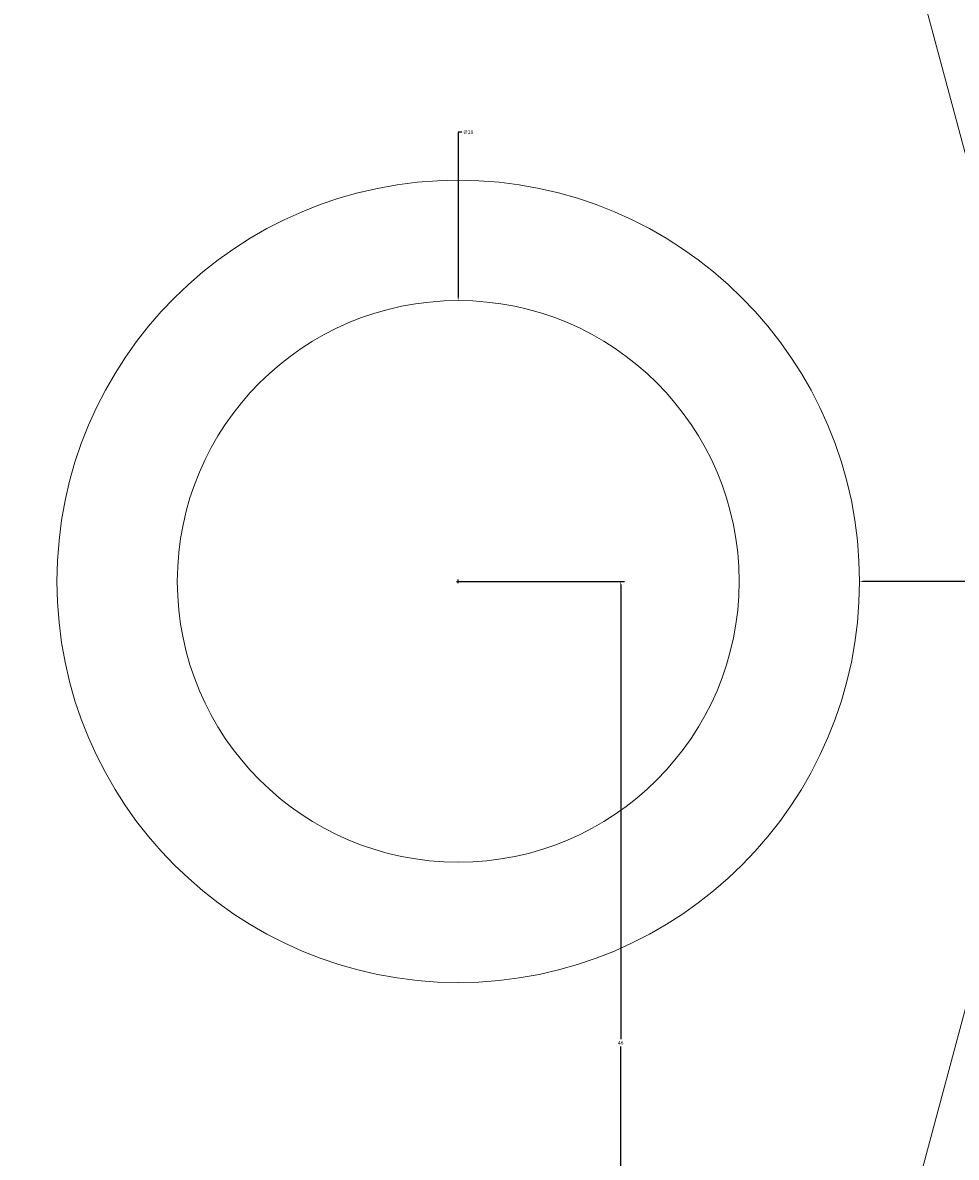
# Model space of a CAD drawing. Units: millimetres. Extents: x 2597 to 2768, y 1809 to 1980.
# Tile 5 of 7: x 2661 to 2708, y 1866 to 1922. Entities that reach past the tile are written whole.
import ezdxf

# ---------------------------------------------------------------- set-up
doc = ezdxf.new("R2010")
doc.units = ezdxf.units.MM
doc.layers.add('M-CONS', color=8, linetype='Continuous', lineweight=18)
doc.layers.add('M-DIMS', color=2, linetype='Continuous', lineweight=18)
doc.styles.get("Standard").update_dxf_attribs({"font": 'arial.ttf'})
doc.dimstyles.get("Standard").update_dxf_attribs({"dimtxt": 0.18, "dimasz": 0.18, "dimexe": 0.18, "dimexo": 0.0625, "dimgap": 0.09, "dimtad": 0, "dimtih": 1, "dimtoh": 1, "dimdec": 4, "dimzin": 0, "dimdsep": 46, "dimtxsty": 'Standard', "dimcen": 0.09, "dimadec": 0, "dimazin": 0, "dimtfac": 1, "dimtdec": 4, "dimtofl": 0, "dimtmove": 0, "dimatfit": 3, "dimfxl": 1, "dimtolj": 1, "dimtzin": 0, "dimarcsym": 0})

# ---------------------------------------------------------------- blocks, each defined once
blk = doc.blocks.new('*D7')
at = {"layer": 'Defpoints', "color": 0, "transparency": 16777216}
for p in [(2682.776, 1894.43), (2682.776, 1848.43), (2690.876, 1848.43)]:
    blk.add_point(p, dxfattribs=at)
at = {"layer": 'M-DIMS', "color": 0, "lineweight": -2, "transparency": 16777216}
for p, q in [((2682.838, 1894.43), (2691.056, 1894.43)), ((2690.876, 1894.25), (2690.876, 1871.612)), ((2690.876, 1848.61), (2690.876, 1871.248)), ((2682.838, 1848.43), (2691.056, 1848.43))]:
    blk.add_line(p, q, dxfattribs=at)
at = {"layer": 'M-DIMS', "color": 0, "transparency": 16777216}
for points in [[(2690.846, 1894.25), (2690.906, 1894.25), (2690.876, 1894.43)], [(2690.846, 1848.61), (2690.906, 1848.61), (2690.876, 1848.43)]]:
    blk.add_solid(points, dxfattribs=at)
at = {"layer": 'M-DIMS', "color": 0, "transparency": 16777216, "insert": (2690.876, 1871.43), "char_height": 0.18, "attachment_point": 5}
blk.add_mtext('\\A1;46', dxfattribs=at)
blk = doc.blocks.new('*D15')
at = {"layer": 'Defpoints', "color": 0, "transparency": 16777216}
for p in [(2662.776, 1894.43), (2702.776, 1894.43)]:
    blk.add_point(p, dxfattribs=at)
at = {"layer": 'M-DIMS', "color": 0, "lineweight": -2, "transparency": 16777216}
for p, q in [((2682.686, 1894.43), (2682.866, 1894.43)), ((2682.776, 1894.34), (2682.776, 1894.52)), ((2714.776, 1894.43), (2702.956, 1894.43))]:
    blk.add_line(p, q, dxfattribs=at)
at = {"layer": 'M-DIMS', "color": 0, "transparency": 16777216}
blk.add_solid([(2702.956, 1894.46), (2702.956, 1894.4), (2702.776, 1894.43)], dxfattribs=at)
at = {"layer": 'M-DIMS', "color": 0, "transparency": 16777216, "insert": (2715.092, 1894.43), "char_height": 0.18, "attachment_point": 5}
blk.add_mtext('\\A1;∅40', dxfattribs=at)
blk = doc.blocks.new('*D16')
at = {"layer": 'Defpoints', "color": 0, "transparency": 16777216}
for p in [(2682.776, 1908.43), (2682.775, 1880.43)]:
    blk.add_point(p, dxfattribs=at)
at = {"layer": 'M-DIMS', "color": 0, "lineweight": -2, "transparency": 16777216}
for p, q in [((2682.956, 1916.83), (2682.776, 1916.83)), ((2682.776, 1916.83), (2682.776, 1908.61)), ((2682.686, 1894.43), (2682.866, 1894.43)), ((2682.776, 1894.34), (2682.776, 1894.52))]:
    blk.add_line(p, q, dxfattribs=at)
at = {"layer": 'M-DIMS', "color": 0, "transparency": 16777216}
blk.add_solid([(2682.746, 1908.61), (2682.806, 1908.61), (2682.776, 1908.43)], dxfattribs=at)
at = {"layer": 'M-DIMS', "color": 0, "transparency": 16777216, "insert": (2683.273, 1916.83), "char_height": 0.18, "attachment_point": 5}
blk.add_mtext('\\A1;∅28', dxfattribs=at)

msp = doc.modelspace()

# ---------------------------------------------------------------- linework, layer by layer
at = {"layer": 'M-CONS'}
msp.add_lwpolyline([(2713.7756, 1903.4301), (2745.7756, 1903.4301), (2745.7756, 1913.4301), (2708.6698, 1913.4301), (2700.1588, 1945.1014, 0.7667514), (2665.3923, 1945.1014), (2656.8814, 1913.4301), (2619.7756, 1913.4301), (2619.7756, 1903.4301), (2651.7756, 1903.4301), (2651.7756, 1885.4301), (2619.7756, 1885.4301), (2619.7756, 1875.4301), (2656.8814, 1875.4301), (2665.3923, 1843.7587, 0.7667514), (2700.1588, 1843.7587), (2708.6698, 1875.4301), (2745.7756, 1875.4301), (2745.7756, 1885.4301), (2713.7756, 1885.4301), (2713.7756, 1903.4301), (2713.7756, 1894.4301)], format="xyb", dxfattribs=at)
for radius in [20, 14]:
    msp.add_circle((2682.7756, 1894.4301), radius, dxfattribs=at)

# ---------------------------------------------------------------- dimensions: what is measured, and where the dimension line sits
at = {"layer": 'M-DIMS'}
for p1, p2, picture, middle in [((2682.7751, 1880.4301), (2682.776, 1908.4301), '*D16', (2683.2733, 1916.8301)), ((2662.7756, 1894.4302), (2702.7756, 1894.43), '*D15', (2714.7756, 1894.4299))]:
    dim = msp.add_diameter_dim_2p(p1=p1, p2=p2, dimstyle='Standard', override={"dimdec": 0, "dimlfac": 1, "dimrnd": 0, "dimzin": 0, "dimdsep": 46, "dimlunit": 2}, dxfattribs=at)
    dim.commit()
    dim.dimension.update_dxf_attribs({"geometry": picture, "text_midpoint": middle, "dimtype": 163})
dim = msp.add_linear_dim(base=(2690.8756, 1848.4301), p1=(2682.7756, 1894.4301), p2=(2682.7756, 1848.4301), angle=270, dimstyle='Standard', override={"dimdec": 0, "dimlfac": 1, "dimrnd": 0, "dimzin": 0, "dimdsep": 46, "dimlunit": 2}, dxfattribs=at)
dim.commit()
dim.dimension.update_dxf_attribs({"geometry": '*D7', "text_midpoint": (2690.8756, 1871.4301)})

doc.saveas('drawing.dxf')
